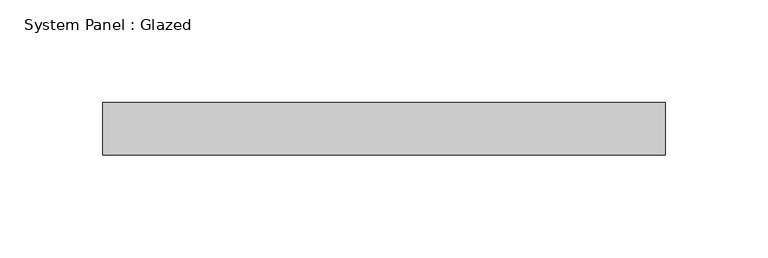
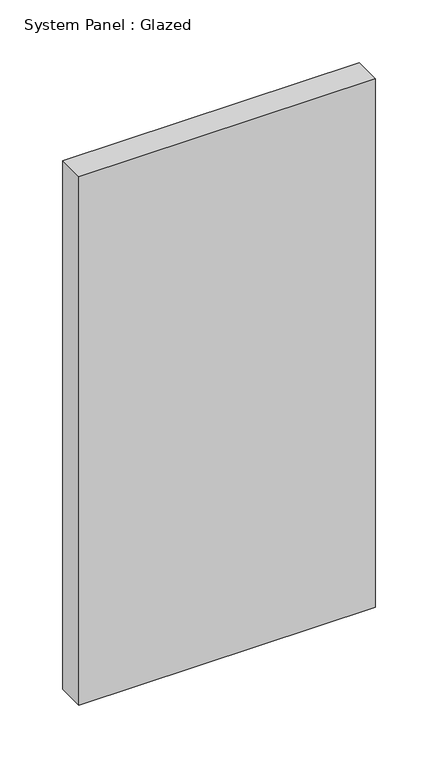
"""IFC4 building model written with IfcOpenShell, lengths in millimetres: plate geometry, System Panel : Glazed."""

from ifc_helpers import new_model, si_unit, origin, origin_with_axes, place, context, project, spatial, polyline, outline, extrude, source, transform, mapped, element, save


def system_panel_glazed_5dcb8e4e(model_context):
    return source(origin(), model_context, "Body", "SweptSolid", [
        extrude(outline(polyline([(136.525, -44.45), (-136.525, -44.45), (-136.525, -19.05), (136.525, -19.05), (136.525, -44.45)])), origin_with_axes(), (0.0, 0.0, 1.0), 514.35),
    ])


if __name__ == "__main__":
    model = new_model("IFC4")
    model_context = context("Model", 3, world=origin())
    ifc_project = project(units=[si_unit("LENGTHUNIT", "METRE", prefix="MILLI")], contexts=[model_context])
    site = spatial("IfcSite", under=ifc_project)
    building = spatial("IfcBuilding", under=site)
    placement = place(None, origin())
    system_panel_glazed_shape = system_panel_glazed_5dcb8e4e(model_context)
    element("IfcPlate", 1, ObjectType="System Panel : Glazed", at=placement, inside=building, context=model_context, shape_type="MappedRepresentation", body=[
        mapped(system_panel_glazed_shape, transform((0.0, 0.0, 0.0), x_axis=(1.0, 0.0, 0.0), y_axis=(0.0, 1.0, 0.0), z_axis=(0.0, 0.0, 1.0))),
    ])
    save(model, "model.ifc")

# Revit data of these elements
# Type "System Panel : Glazed"
#   Construction Type Id = "GSP4R"
#   Analytic Construction = "1/8 in Pilkington single glazing"
#   Visual Light Transmittance = 0.9
#   Solar Heat Gain Coefficient = 0.86
#   Heat Transfer Coefficient (U) = 1.18115 BTU/(h·ft²·°F)
# Element 1 (IfcPlate, "System Panel : Glazed")
#   Materials on its faces: "Glass"
# Materials
#   "Glass": class "Glass", colour RGB 0 128 192, transparency 0.75, Description = "Soda Lime Glass", Cost = 0
